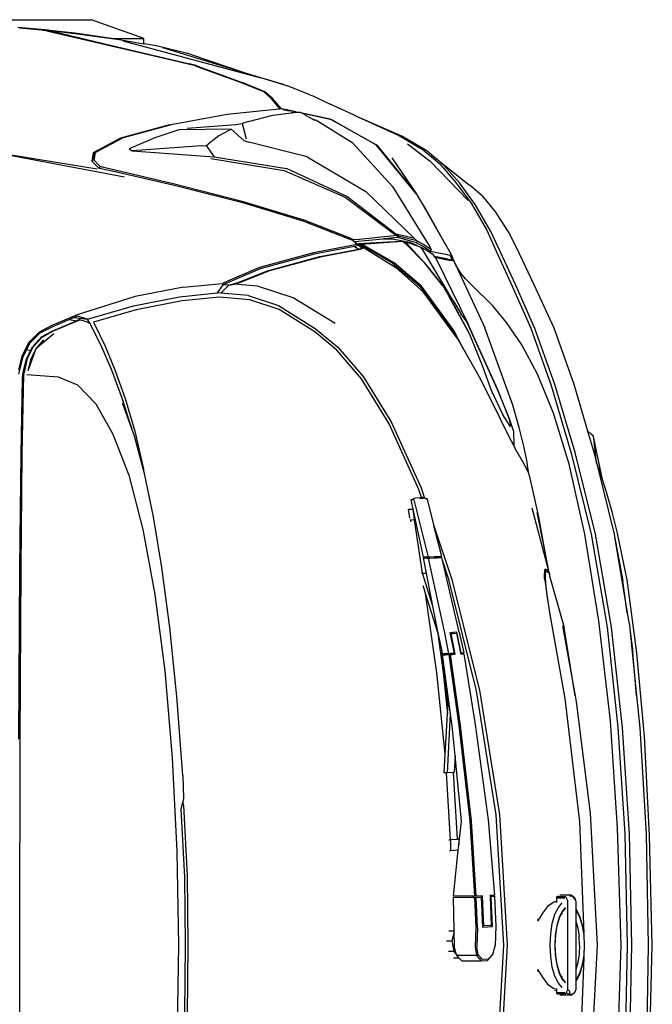
# Model space of a CAD drawing. Units: inches. Extents: x 22042254 to 25404563, y 17568978 to 17626777.
# Tile 18 of 45: x 22042342.8522 to 22042343.228, y 17568978.1821 to 17568978.767. Entities that reach past the tile are written whole.
import ezdxf

# ---------------------------------------------------------------- set-up
doc = ezdxf.new("R2010")
doc.units = ezdxf.units.IN
doc.header["$MEASUREMENT"] = 0
doc.layers.add('A-SITE-VEHI', color=8, linetype='Continuous', lineweight=18)
doc.layers.add('Edges', color=250, linetype='Continuous')

# ---------------------------------------------------------------- blocks, each defined once
blk = doc.blocks.new('Nissan Qashqai pl')
at = {"layer": 'Edges'}
for p, q in [((11.05972, 12.11965), (11.05938, 11.92208)), ((11.5166, 12.04708), (11.52386, 11.92208)), ((11.52698, 11.92208), (11.51964, 12.0475)), ((11.61327, 11.92208), (11.60675, 12.04892)), ((11.60051, 11.93346), (11.59629, 12.04057)), ((11.63292, 12.0344), (11.63628, 11.92208)), ((11.64211, 11.92208), (11.63993, 12.02899)), ((11.64437, 12.02886), (11.64655, 11.92208)), ((11.66226, 11.92208), (11.66041, 12.02874)), ((11.66349, 12.02738), (11.66628, 11.92208)), ((11.21164, 11.92208), (11.21014, 12.01197)), ((11.22044, 11.98904), (11.22108, 11.92208)), ((11.21801, 11.92208), (11.21745, 11.98742)), ((11.57617, 11.96938), (11.57479, 11.96843)), ((11.58846, 11.97008), (11.57758, 11.97008)), ((11.58668, 11.96947), (11.58377, 11.96782)), ((11.58679, 11.96604), (11.58668, 11.96947)), ((11.58961, 11.96947), (11.58668, 11.96947)), ((11.58846, 11.97008), (11.58961, 11.96947)), ((11.5915, 11.96782), (11.58961, 11.96947)), ((11.56588, 11.95938), (11.57195, 11.96347)), ((11.57195, 11.96347), (11.57457, 11.96395)), ((11.57261, 11.96533), (11.57261, 11.96561)), ((11.57306, 11.96528), (11.57306, 11.96569)), ((11.57479, 11.96843), (11.57457, 11.96768)), ((11.58239, 11.96768), (11.57457, 11.96768)), ((11.57457, 11.96768), (11.57457, 11.96395)), ((11.57457, 11.96395), (11.57457, 11.96378)), ((11.57479, 11.96843), (11.58262, 11.96843)), ((11.57994, 11.96265), (11.57613, 11.95845)), ((11.58262, 11.96843), (11.58377, 11.96782)), ((11.58377, 11.96782), (11.58513, 11.96453)), ((11.58679, 11.96604), (11.58513, 11.96453)), ((11.58513, 11.96453), (11.58513, 11.87963)), ((11.5915, 11.96782), (11.59043, 11.96839)), ((11.59285, 11.96453), (11.5915, 11.96782)), ((11.59285, 11.95694), (11.59285, 11.96453)), ((11.55816, 11.94815), (11.56082, 11.95281)), ((11.56082, 11.95281), (11.56588, 11.95938)), ((11.57286, 11.95178), (11.57035, 11.94308)), ((11.57613, 11.95845), (11.57286, 11.95178)), ((11.57692, 11.94885), (11.57987, 11.95487)), ((11.57876, 11.95169), (11.57712, 11.94834)), ((11.58001, 11.95424), (11.57876, 11.95169)), ((11.57876, 11.95169), (11.57995, 11.953)), ((11.57987, 11.95487), (11.58291, 11.95821)), ((11.58291, 11.95743), (11.58001, 11.95424)), ((11.59285, 11.95694), (11.59412, 11.95487)), ((11.59285, 11.95657), (11.59285, 11.95694)), ((11.59319, 11.9559), (11.59285, 11.95657)), ((11.59285, 11.95626), (11.59285, 11.95657)), ((11.59285, 11.95626), (11.59319, 11.9559)), ((11.59285, 11.95549), (11.59285, 11.95626)), ((11.59398, 11.95424), (11.59285, 11.95549)), ((11.59285, 11.94526), (11.59285, 11.95549)), ((11.59319, 11.9559), (11.59412, 11.95487)), ((11.59688, 11.94834), (11.59398, 11.95424)), ((11.59412, 11.95487), (11.59707, 11.94885)), ((11.55654, 11.94509), (11.55639, 11.94749)), ((11.55654, 11.94509), (11.55816, 11.94815)), ((11.57035, 11.94308), (11.56877, 11.93295)), ((11.57324, 11.93188), (11.57466, 11.94101)), ((11.5749, 11.94065), (11.5735, 11.93169)), ((11.57466, 11.94101), (11.57692, 11.94885)), ((11.57712, 11.94834), (11.5749, 11.94065)), ((11.59285, 11.8989), (11.59285, 11.94526)), ((11.59478, 11.93858), (11.59285, 11.94526)), ((11.5991, 11.94065), (11.59688, 11.94834)), ((11.59707, 11.94885), (11.59933, 11.94101)), ((11.60049, 11.93169), (11.5991, 11.94065)), ((11.59933, 11.94101), (11.60051, 11.93346)), ((11.48106, 11.93457), (11.47554, 11.93456)), ((11.47578, 11.92803), (11.4784, 11.93124)), ((11.4784, 11.93124), (11.47657, 11.92368)), ((11.4786, 11.93206), (11.4784, 11.93124)), ((11.48106, 11.93457), (11.4786, 11.93206)), ((11.49744, 11.93207), (11.4786, 11.93206)), ((11.48349, 11.93703), (11.48106, 11.93457)), ((11.48349, 11.93703), (11.50222, 11.93704)), ((11.49621, 11.92369), (11.49744, 11.93207)), ((11.49744, 11.93207), (11.50222, 11.93704)), ((11.49907, 11.93132), (11.49795, 11.92364)), ((11.50349, 11.93588), (11.49907, 11.93132)), ((11.50222, 11.93704), (11.50812, 11.93671)), ((11.50889, 11.93558), (11.50349, 11.93588)), ((11.50812, 11.93671), (11.51287, 11.9312)), ((11.50889, 11.93558), (11.51321, 11.93053)), ((11.51321, 11.93053), (11.51287, 11.9312)), ((11.56877, 11.93295), (11.56823, 11.92208)), ((11.57275, 11.92208), (11.57324, 11.93188)), ((11.5735, 11.93169), (11.57302, 11.92208)), ((11.59602, 11.93062), (11.59478, 11.93858)), ((11.60097, 11.92208), (11.60049, 11.93169)), ((11.60051, 11.93346), (11.60076, 11.93188)), ((11.60076, 11.93188), (11.60124, 11.92208)), ((11.05938, 11.92208), (11.05972, 11.72451)), ((11.21014, 11.8322), (11.21164, 11.92208)), ((11.21745, 11.85674), (11.21801, 11.92208)), ((11.22108, 11.92208), (11.22044, 11.85512)), ((11.47578, 11.92803), (11.47062, 11.92803)), ((11.47398, 11.91798), (11.47578, 11.92803)), ((11.47657, 11.92368), (11.47622, 11.90912)), ((11.49689, 11.90495), (11.49621, 11.92369)), ((11.49859, 11.9049), (11.49795, 11.92364)), ((11.51321, 11.93053), (11.51543, 11.92267)), ((11.51606, 11.90392), (11.51543, 11.92267)), ((11.52386, 11.92208), (11.5166, 11.79708)), ((11.51964, 11.79666), (11.52698, 11.92208)), ((11.56823, 11.92208), (11.56877, 11.91121)), ((11.57324, 11.91228), (11.57275, 11.92208)), ((11.57302, 11.92208), (11.5735, 11.91247)), ((11.59645, 11.92208), (11.59602, 11.93062)), ((11.59645, 11.92208), (11.59602, 11.91354)), ((11.60049, 11.91247), (11.60097, 11.92208)), ((11.60124, 11.92208), (11.60076, 11.91228)), ((11.60675, 11.79524), (11.61327, 11.92208)), ((11.63628, 11.92208), (11.63292, 11.80976)), ((11.63993, 11.81518), (11.64211, 11.92208)), ((11.64655, 11.92208), (11.64437, 11.8153)), ((11.66041, 11.81542), (11.66226, 11.92208)), ((11.66628, 11.92208), (11.66349, 11.81678)), ((11.46896, 11.91798), (11.47398, 11.91798)), ((11.47622, 11.90912), (11.47398, 11.91798)), ((11.57466, 11.90315), (11.57324, 11.91228)), ((11.5735, 11.91247), (11.5749, 11.90351)), ((11.59478, 11.90558), (11.59602, 11.91354)), ((11.5991, 11.90351), (11.60049, 11.91247)), ((11.60076, 11.91228), (11.60051, 11.91071)), ((11.47102, 11.90825), (11.4762, 11.90826)), ((11.4762, 11.90826), (11.47542, 11.87608)), ((11.47622, 11.90912), (11.4762, 11.90826)), ((11.49565, 11.87616), (11.49689, 11.90495)), ((11.49859, 11.9049), (11.49735, 11.87612)), ((11.50223, 11.8759), (11.50346, 11.90468)), ((11.50462, 11.90341), (11.50341, 11.87505)), ((11.50346, 11.90468), (11.51299, 11.90415)), ((11.51177, 11.90301), (11.50462, 11.90341)), ((11.51058, 11.87508), (11.51177, 11.90301)), ((11.51299, 11.90415), (11.51176, 11.87537)), ((11.51483, 11.87514), (11.51606, 11.90392)), ((11.56877, 11.91121), (11.57035, 11.90108)), ((11.57692, 11.89531), (11.57466, 11.90315)), ((11.5749, 11.90351), (11.57712, 11.89582)), ((11.59285, 11.8989), (11.59478, 11.90558)), ((11.59629, 11.80359), (11.60051, 11.91071)), ((11.59688, 11.89582), (11.5991, 11.90351)), ((11.59933, 11.90315), (11.59707, 11.89531)), ((11.60051, 11.91071), (11.59933, 11.90315)), ((11.55639, 11.89667), (11.55654, 11.89907)), ((11.55816, 11.89601), (11.55654, 11.89907)), ((11.56082, 11.89135), (11.55816, 11.89601)), ((11.57035, 11.90108), (11.57286, 11.89238)), ((11.57987, 11.88929), (11.57692, 11.89531)), ((11.57712, 11.89582), (11.57876, 11.89248)), ((11.59285, 11.88868), (11.59285, 11.8989)), ((11.59398, 11.88992), (11.59688, 11.89582)), ((11.59707, 11.89531), (11.59412, 11.88929)), ((11.56588, 11.88478), (11.56082, 11.89135)), ((11.57195, 11.88069), (11.56588, 11.88478)), ((11.57286, 11.89238), (11.57613, 11.88571)), ((11.57613, 11.88571), (11.57994, 11.88151)), ((11.57995, 11.89116), (11.57876, 11.89248)), ((11.57876, 11.89248), (11.58001, 11.88992)), ((11.58291, 11.88595), (11.57987, 11.88929)), ((11.58001, 11.88992), (11.58291, 11.88673)), ((11.59285, 11.88868), (11.59398, 11.88992)), ((11.59285, 11.88722), (11.59412, 11.88929)), ((11.59285, 11.8879), (11.59285, 11.88868)), ((11.59285, 11.88759), (11.59319, 11.88827)), ((11.59319, 11.88827), (11.59285, 11.8879)), ((11.59285, 11.88759), (11.59285, 11.8879)), ((11.59285, 11.88722), (11.59285, 11.88759)), ((11.59285, 11.87963), (11.59285, 11.88722)), ((11.59412, 11.88929), (11.59319, 11.88827)), ((11.49563, 11.87496), (11.47539, 11.87488)), ((11.47539, 11.87488), (11.4801, 11.83099)), ((11.47542, 11.87608), (11.49451, 11.87616)), ((11.49133, 11.80278), (11.49563, 11.87496)), ((11.49732, 11.87492), (11.49295, 11.80271)), ((11.49449, 11.87502), (11.49451, 11.87616)), ((11.50341, 11.87505), (11.49449, 11.87502)), ((11.49451, 11.87616), (11.49565, 11.87616)), ((11.49732, 11.87492), (11.49563, 11.87496)), ((11.49565, 11.87616), (11.49735, 11.87612)), ((11.50339, 11.87463), (11.49732, 11.87492)), ((11.49735, 11.87612), (11.50223, 11.8759)), ((11.50341, 11.87505), (11.50339, 11.87463)), ((11.51054, 11.87423), (11.51058, 11.87508)), ((11.51472, 11.8751), (11.51058, 11.87508)), ((11.51176, 11.87537), (11.51472, 11.87515)), ((11.51472, 11.87515), (11.51472, 11.8751)), ((11.51472, 11.87515), (11.51483, 11.87514)), ((11.51483, 11.87514), (11.51472, 11.8751)), ((11.57261, 11.88057), (11.57195, 11.88069)), ((11.57261, 11.88057), (11.57261, 11.88076)), ((11.57306, 11.88049), (11.57261, 11.88057)), ((11.57306, 11.88049), (11.57306, 11.88081)), ((11.57457, 11.88021), (11.57306, 11.88049)), ((11.57457, 11.88096), (11.57457, 11.88021)), ((11.57457, 11.88021), (11.57457, 11.87648)), ((11.57457, 11.87648), (11.58239, 11.87648)), ((11.57457, 11.87648), (11.57479, 11.87573)), ((11.58262, 11.87573), (11.57479, 11.87573)), ((11.57479, 11.87573), (11.57617, 11.87478)), ((11.58377, 11.87635), (11.58262, 11.87573)), ((11.58513, 11.87963), (11.58377, 11.87635)), ((11.58668, 11.87469), (11.58961, 11.87469)), ((11.58961, 11.87469), (11.58846, 11.87408)), ((11.58961, 11.87469), (11.5915, 11.87635)), ((11.59043, 11.87577), (11.58961, 11.87469)), ((11.59221, 11.87812), (11.59043, 11.87577)), ((11.59043, 11.87577), (11.5915, 11.87635)), ((11.5915, 11.87635), (11.59221, 11.87812)), ((11.59285, 11.87963), (11.59221, 11.87812)), ((11.50884, 11.80182), (11.5148, 11.87394)), ((11.5148, 11.87394), (11.51054, 11.87423)), ((11.58846, 11.87408), (11.57758, 11.87408)), ((11.2139, 11.7914), (11.21745, 11.85674)), ((11.22044, 11.85512), (11.21682, 11.78816)), ((11.20565, 11.74231), (11.21014, 11.8322)), ((11.47305, 11.83139), (11.47165, 11.83144)), ((11.47305, 11.83139), (11.473, 11.82087)), ((11.4801, 11.83099), (11.47305, 11.83139)), ((11.4801, 11.83099), (11.48065, 11.82584)), ((11.47281, 11.82086), (11.46872, 11.75675)), ((11.47111, 11.82093), (11.47189, 11.82089)), ((11.47281, 11.82086), (11.47189, 11.82089)), ((11.473, 11.82087), (11.47281, 11.82086)), ((11.47916, 11.8205), (11.473, 11.82087)), ((11.47508, 11.75641), (11.47919, 11.82046)), ((11.47919, 11.82046), (11.47916, 11.8205)), ((11.48062, 11.82044), (11.47919, 11.82046)), ((11.48062, 11.82044), (11.48065, 11.82584)), ((11.48065, 11.82584), (11.4831, 11.803)), ((11.63292, 11.80976), (11.62604, 11.70665)), ((11.63327, 11.71316), (11.63993, 11.81518)), ((11.64437, 11.8153), (11.63768, 11.7134)), ((11.65425, 11.71357), (11.66041, 11.81542)), ((11.66349, 11.81678), (11.65888, 11.72193)), ((11.4831, 11.803), (11.47707, 11.74042)), ((11.4805, 11.71128), (11.49133, 11.80278)), ((11.49295, 11.80271), (11.48212, 11.71121)), ((11.49642, 11.71041), (11.50884, 11.80182)), ((11.58235, 11.68521), (11.59629, 11.80359)), ((11.21579, 11.78424), (11.2139, 11.7914)), ((11.5166, 11.79708), (11.49761, 11.67796)), ((11.50045, 11.6772), (11.51964, 11.79666)), ((11.5932, 11.68852), (11.60675, 11.79524)), ((11.21682, 11.78816), (11.21579, 11.78424)), ((11.21585, 11.78401), (11.21579, 11.78424)), ((11.21682, 11.78816), (11.21585, 11.78401)), ((11.21658, 11.78121), (11.21585, 11.78401)), ((11.21586, 11.75915), (11.21658, 11.78121)), ((11.21586, 11.75915), (11.20997, 11.68347)), ((11.46872, 11.75675), (11.46649, 11.75682)), ((11.46649, 11.75682), (11.46757, 11.73891)), ((11.46975, 11.75671), (11.46872, 11.75675)), ((11.46975, 11.75671), (11.47273, 11.69994)), ((11.47508, 11.75641), (11.46975, 11.75671)), ((11.47611, 11.75636), (11.47508, 11.75641)), ((11.47707, 11.74042), (11.47611, 11.75636)), ((11.19842, 11.65867), (11.20565, 11.74231)), ((11.46757, 11.73891), (11.45941, 11.6607)), ((11.46757, 11.73891), (11.46992, 11.70014)), ((11.47707, 11.74042), (11.47428, 11.71144)), ((11.0586, 11.72441), (11.05947, 11.55994)), ((11.05972, 11.72451), (11.06059, 11.56009)), ((11.65888, 11.72193), (11.65143, 11.64152)), ((11.47094, 11.64327), (11.4805, 11.71128)), ((11.48212, 11.71121), (11.47257, 11.6432)), ((11.47428, 11.71144), (11.47273, 11.69994)), ((11.48539, 11.64249), (11.49642, 11.71041)), ((11.62604, 11.70665), (11.61495, 11.61084)), ((11.6229, 11.61679), (11.63327, 11.71316)), ((11.63768, 11.7134), (11.62719, 11.61693)), ((11.65114, 11.68233), (11.65425, 11.71357)), ((11.47273, 11.69994), (11.46512, 11.64343)), ((11.46576, 11.66035), (11.46992, 11.70014)), ((11.46992, 11.70014), (11.47047, 11.69095)), ((11.47047, 11.69095), (11.46419, 11.63849)), ((11.59218, 11.68277), (11.5932, 11.68852)), ((11.20997, 11.68347), (11.2033, 11.61723)), ((11.49761, 11.67796), (11.47115, 11.57128)), ((11.47375, 11.5702), (11.50045, 11.6772)), ((11.56846, 11.60829), (11.58235, 11.68521)), ((11.58021, 11.61555), (11.59218, 11.68277)), ((11.59218, 11.68277), (11.58179, 11.61717)), ((11.64478, 11.61839), (11.65114, 11.68233)), ((11.65114, 11.68233), (11.64749, 11.64092)), ((11.18907, 11.58559), (11.19842, 11.65867)), ((11.45941, 11.6607), (11.44866, 11.58459)), ((11.46024, 11.62121), (11.46576, 11.66035)), ((11.46419, 11.63849), (11.46114, 11.62406)), ((11.46505, 11.64255), (11.46419, 11.63849)), ((11.46792, 11.64248), (11.46505, 11.64255)), ((11.46512, 11.64343), (11.46801, 11.64335)), ((11.46687, 11.62247), (11.47088, 11.64239)), ((11.46801, 11.64335), (11.46792, 11.64248)), ((11.47088, 11.64239), (11.46792, 11.64248)), ((11.46801, 11.64335), (11.47094, 11.64327)), ((11.47252, 11.64233), (11.47088, 11.64239)), ((11.47094, 11.64327), (11.47257, 11.6432)), ((11.47212, 11.62223), (11.47625, 11.64214)), ((11.47439, 11.64223), (11.47252, 11.64233)), ((11.47257, 11.6432), (11.47449, 11.6431)), ((11.47727, 11.64296), (11.47315, 11.62305)), ((11.47439, 11.64223), (11.47449, 11.6431)), ((11.47625, 11.64214), (11.47439, 11.64223)), ((11.47449, 11.6431), (11.47727, 11.64296)), ((11.47827, 11.62277), (11.48226, 11.64167)), ((11.48298, 11.64165), (11.47879, 11.62186)), ((11.48098, 11.62171), (11.48532, 11.64161)), ((11.48226, 11.64167), (11.48244, 11.64254)), ((11.48226, 11.64167), (11.48298, 11.64165)), ((11.48244, 11.64254), (11.48247, 11.64267)), ((11.48535, 11.64246), (11.48244, 11.64254)), ((11.48247, 11.64267), (11.48535, 11.64246)), ((11.483, 11.64176), (11.48298, 11.64165)), ((11.48532, 11.64161), (11.483, 11.64176)), ((11.48539, 11.64249), (11.48535, 11.64246)), ((11.65143, 11.64152), (11.64217, 11.57162)), ((11.64478, 11.61839), (11.64749, 11.64092)), ((11.46024, 11.62121), (11.44866, 11.58459)), ((11.45125, 11.55073), (11.46687, 11.62247)), ((11.46083, 11.62261), (11.45585, 11.5969)), ((11.46114, 11.62406), (11.46024, 11.62121)), ((11.46114, 11.62406), (11.46083, 11.62261)), ((11.48098, 11.62171), (11.4649, 11.55261)), ((11.47495, 11.62207), (11.47212, 11.62223)), ((11.47315, 11.62305), (11.47515, 11.62294)), ((11.47495, 11.62207), (11.47515, 11.62294)), ((11.47879, 11.62186), (11.47495, 11.62207)), ((11.47515, 11.62294), (11.47827, 11.62277)), ((11.2033, 11.61723), (11.19582, 11.55976)), ((11.56776, 11.56755), (11.58179, 11.61717)), ((11.61495, 11.61084), (11.6016, 11.52761)), ((11.60765, 11.5276), (11.6229, 11.61679)), ((11.62719, 11.61693), (11.61178, 11.52762)), ((11.64227, 11.603), (11.64462, 11.61709)), ((11.64462, 11.61709), (11.64478, 11.61839)), ((11.56499, 11.58644), (11.56846, 11.60829)), ((11.56905, 11.60888), (11.56563, 11.58822)), ((11.63012, 11.53004), (11.64227, 11.603)), ((11.64227, 11.603), (11.63807, 11.5726)), ((11.45585, 11.5969), (11.44582, 11.56516)), ((11.45585, 11.5969), (11.44965, 11.56495)), ((11.17758, 11.52307), (11.18907, 11.58559)), ((11.44866, 11.58459), (11.44723, 11.58007)), ((11.56356, 11.57357), (11.56499, 11.58644)), ((11.56563, 11.58822), (11.56415, 11.57536)), ((11.44723, 11.58007), (11.44639, 11.57739)), ((11.56335, 11.56843), (11.56356, 11.57357)), ((11.56415, 11.57536), (11.56375, 11.56794)), ((11.63012, 11.53004), (11.63807, 11.5726)), ((11.44575, 11.56516), (11.43801, 11.51398)), ((11.4448, 11.5652), (11.44575, 11.56516)), ((11.44575, 11.56516), (11.44582, 11.56516)), ((11.44582, 11.56516), (11.44965, 11.56495)), ((11.44965, 11.56495), (11.44685, 11.5505)), ((11.45676, 11.51971), (11.47375, 11.5702)), ((11.47115, 11.57128), (11.4649, 11.55261)), ((11.56255, 11.56701), (11.56268, 11.56956)), ((11.56271, 11.56245), (11.56255, 11.56701)), ((11.56268, 11.56956), (11.56259, 11.5697)), ((11.56268, 11.56956), (11.5628, 11.57206)), ((11.56335, 11.56843), (11.56268, 11.56956)), ((11.56325, 11.56586), (11.56335, 11.56843)), ((11.56334, 11.56271), (11.56325, 11.56586)), ((11.56609, 11.56386), (11.56334, 11.56271)), ((11.56368, 11.56788), (11.56335, 11.56843)), ((11.56375, 11.56794), (11.56392, 11.56325)), ((11.56392, 11.56325), (11.56429, 11.56338)), ((11.56429, 11.56338), (11.56596, 11.56408)), ((11.56487, 11.5659), (11.56469, 11.5662)), ((11.56609, 11.56386), (11.56583, 11.56223)), ((11.56596, 11.56408), (11.56616, 11.56417)), ((11.56609, 11.56386), (11.56596, 11.56408)), ((11.56613, 11.56388), (11.56609, 11.56386)), ((11.56618, 11.56418), (11.56613, 11.56388)), ((11.56613, 11.56388), (11.56616, 11.56417)), ((11.56613, 11.56388), (11.56645, 11.5641)), ((11.56665, 11.56424), (11.56616, 11.56236)), ((11.56616, 11.56417), (11.56618, 11.56418)), ((11.56616, 11.56236), (11.56645, 11.5641)), ((11.56618, 11.56418), (11.56648, 11.56431)), ((11.56645, 11.5641), (11.56648, 11.56431)), ((11.56645, 11.5641), (11.56665, 11.56424)), ((11.56648, 11.56431), (11.56669, 11.5644)), ((11.56661, 11.56253), (11.56704, 11.56455)), ((11.56665, 11.56424), (11.56688, 11.56448)), ((11.56669, 11.5644), (11.56665, 11.56424)), ((11.56669, 11.5644), (11.56688, 11.56448)), ((11.56671, 11.56257), (11.56712, 11.56458)), ((11.56717, 11.5646), (11.56679, 11.56261)), ((11.56688, 11.56448), (11.56704, 11.56455)), ((11.56704, 11.56455), (11.56739, 11.56625)), ((11.56704, 11.56455), (11.56712, 11.56458)), ((11.56712, 11.56458), (11.56763, 11.56708)), ((11.56712, 11.56458), (11.56717, 11.5646)), ((11.56717, 11.5646), (11.56763, 11.56708)), ((11.56745, 11.56646), (11.56739, 11.56625)), ((11.56763, 11.56708), (11.56776, 11.56755)), ((11.64217, 11.57162), (11.63751, 11.54857)), ((11.05947, 11.55994), (11.06074, 11.45082)), ((11.06059, 11.56009), (11.06182, 11.4509)), ((11.19582, 11.55976), (11.18773, 11.51111)), ((11.55053, 11.5023), (11.56648, 11.56144)), ((11.56334, 11.56271), (11.56271, 11.56245)), ((11.56338, 11.56129), (11.56271, 11.56245)), ((11.56273, 11.5431), (11.56648, 11.56144)), ((11.56338, 11.56129), (11.56334, 11.56271)), ((11.56583, 11.56223), (11.56338, 11.56129)), ((11.56616, 11.56236), (11.56583, 11.56223)), ((11.56661, 11.56253), (11.56616, 11.56236)), ((11.56679, 11.56261), (11.56648, 11.56144)), ((11.56671, 11.56257), (11.56661, 11.56253)), ((11.56679, 11.56261), (11.56671, 11.56257)), ((11.43747, 11.49463), (11.45125, 11.54985)), ((11.44684, 11.54963), (11.43914, 11.51392)), ((11.44983, 11.54978), (11.44684, 11.54963)), ((11.44685, 11.5505), (11.44997, 11.55066)), ((11.44983, 11.54978), (11.44997, 11.55066)), ((11.45125, 11.54985), (11.44983, 11.54978)), ((11.44997, 11.55066), (11.45125, 11.55073)), ((11.45125, 11.55073), (11.4529, 11.55066)), ((11.4529, 11.54978), (11.45125, 11.54985)), ((11.4529, 11.55066), (11.45711, 11.55045)), ((11.45711, 11.54958), (11.4529, 11.54978)), ((11.46429, 11.54915), (11.45676, 11.51971)), ((11.45711, 11.55045), (11.45994, 11.5503)), ((11.46197, 11.5493), (11.45711, 11.54958)), ((11.45983, 11.54978), (11.45994, 11.5503)), ((11.46402, 11.54999), (11.45983, 11.54978)), ((11.45994, 11.5503), (11.46197, 11.55018)), ((11.46197, 11.55018), (11.46404, 11.55004)), ((11.46375, 11.54918), (11.46197, 11.5493)), ((11.46402, 11.54999), (11.46375, 11.54918)), ((11.46429, 11.54915), (11.46375, 11.54918)), ((11.46404, 11.55004), (11.46402, 11.54999)), ((11.46423, 11.55), (11.46402, 11.54999)), ((11.46404, 11.55004), (11.46423, 11.55)), ((11.46423, 11.55), (11.46424, 11.55003)), ((11.4643, 11.55002), (11.46423, 11.55)), ((11.4649, 11.55261), (11.4643, 11.55002)), ((11.63751, 11.54857), (11.63276, 11.52672)), ((11.55533, 11.50682), (11.56273, 11.5431)), ((11.55707, 11.51104), (11.56273, 11.5431)), ((11.6016, 11.52761), (11.58664, 11.46068)), ((11.58843, 11.44985), (11.60765, 11.5276)), ((11.61178, 11.52762), (11.59225, 11.44945)), ((11.61272, 11.45895), (11.62966, 11.52759)), ((11.63276, 11.52672), (11.62771, 11.50627)), ((11.62966, 11.52759), (11.63012, 11.53004)), ((11.16395, 11.47112), (11.17758, 11.52307)), ((11.43501, 11.51584), (11.43475, 11.51409)), ((11.45032, 11.49453), (11.45676, 11.51971)), ((11.18773, 11.51111), (11.17906, 11.46956)), ((11.43371, 11.51238), (11.43251, 11.50378)), ((11.43475, 11.51409), (11.43403, 11.51411)), ((11.43801, 11.51398), (11.43475, 11.51409)), ((11.4382, 11.51397), (11.43676, 11.50364)), ((11.43914, 11.51392), (11.43692, 11.50363)), ((11.4382, 11.51397), (11.43801, 11.51398)), ((11.43914, 11.51392), (11.4382, 11.51397)), ((11.54814, 11.47101), (11.55707, 11.51104)), ((11.62771, 11.50627), (11.62241, 11.48743)), ((11.43251, 11.50378), (11.43676, 11.50364)), ((11.43251, 11.50378), (11.4369, 11.50353)), ((11.4369, 11.50353), (11.435, 11.49469)), ((11.43676, 11.50364), (11.43692, 11.50363)), ((11.43692, 11.50363), (11.4369, 11.50353)), ((11.435, 11.49469), (11.43896, 11.49272)), ((11.43747, 11.49463), (11.435, 11.49469)), ((11.43896, 11.49272), (11.44373, 11.49245)), ((11.44474, 11.49242), (11.44218, 11.48476)), ((11.44507, 11.49341), (11.44316, 11.49351)), ((11.44373, 11.49245), (11.44491, 11.49291)), ((11.44474, 11.49242), (11.44373, 11.49245)), ((11.44453, 11.48334), (11.44778, 11.49299)), ((11.44491, 11.49291), (11.44474, 11.49242)), ((11.4462, 11.49239), (11.44474, 11.49242)), ((11.44507, 11.49341), (11.44491, 11.49291)), ((11.44491, 11.49291), (11.44606, 11.49335)), ((11.44606, 11.49335), (11.44507, 11.49341)), ((11.44786, 11.49325), (11.44606, 11.49335)), ((11.44786, 11.49325), (11.4462, 11.49239)), ((11.44778, 11.49299), (11.4462, 11.49239)), ((11.45018, 11.49392), (11.44778, 11.49299)), ((11.44794, 11.49325), (11.44786, 11.49325)), ((11.45032, 11.49453), (11.44794, 11.49325)), ((11.45018, 11.49392), (11.45032, 11.49453)), ((11.62241, 11.48743), (11.61848, 11.47528)), ((11.44218, 11.48476), (11.41383, 11.42186)), ((11.41588, 11.41997), (11.44453, 11.48334)), ((11.14869, 11.43161), (11.16395, 11.47112)), ((11.17906, 11.46956), (11.17808, 11.46592)), ((11.54554, 11.46484), (11.54721, 11.46841)), ((11.54814, 11.47101), (11.54666, 11.46197)), ((11.61848, 11.47528), (11.61008, 11.43562)), ((11.61742, 11.47198), (11.61272, 11.45895)), ((11.61848, 11.47528), (11.61742, 11.47198)), ((11.17808, 11.46592), (11.1694, 11.43374)), ((11.1699, 11.42889), (11.17797, 11.4652)), ((11.17797, 11.4652), (11.17808, 11.46592)), ((11.54162, 11.45783), (11.54554, 11.46484)), ((11.54666, 11.46197), (11.54611, 11.45874)), ((11.58664, 11.46068), (11.57152, 11.41151)), ((11.61272, 11.45895), (11.61008, 11.43562)), ((11.61028, 11.44915), (11.61272, 11.45895)), ((11.06074, 11.45082), (11.06214, 11.37845)), ((11.06182, 11.4509), (11.06324, 11.37414)), ((11.53572, 11.44731), (11.54162, 11.45783)), ((11.54611, 11.45874), (11.54336, 11.44449)), ((11.56912, 11.38501), (11.58843, 11.44985)), ((11.59225, 11.44945), (11.57263, 11.38419)), ((11.52833, 11.43321), (11.53335, 11.4428)), ((11.53261, 11.43965), (11.5333, 11.44225)), ((11.53313, 11.42848), (11.53354, 11.44315)), ((11.5333, 11.44225), (11.53335, 11.4428)), ((11.53335, 11.4428), (11.53354, 11.44315)), ((11.53354, 11.44315), (11.53572, 11.44731)), ((11.54336, 11.44449), (11.53855, 11.42543)), ((11.60419, 11.42861), (11.61028, 11.44915)), ((11.1323, 11.40268), (11.14869, 11.43161)), ((11.1694, 11.43374), (11.1668, 11.42651)), ((11.5202, 11.41712), (11.52833, 11.43321)), ((11.60772, 11.43162), (11.60419, 11.42861)), ((11.60938, 11.43347), (11.60772, 11.43162)), ((11.61008, 11.43562), (11.60938, 11.43347)), ((11.1668, 11.42651), (11.1582, 11.40259)), ((11.16047, 11.39766), (11.1699, 11.42889)), ((11.16426, 11.41918), (11.1668, 11.42651)), ((11.41383, 11.42186), (11.38718, 11.37878)), ((11.53009, 11.42439), (11.52299, 11.41307)), ((11.52855, 11.41625), (11.53022, 11.42324)), ((11.53313, 11.42848), (11.52922, 11.417)), ((11.53022, 11.42324), (11.53009, 11.42439)), ((11.53855, 11.42543), (11.53253, 11.4038)), ((11.59084, 11.38361), (11.60419, 11.42861)), ((11.15764, 11.39828), (11.16426, 11.41918)), ((11.15766, 11.39771), (11.16426, 11.41918)), ((11.16426, 11.41918), (11.15826, 11.40186)), ((11.38877, 11.37638), (11.41588, 11.41997)), ((11.50131, 11.37908), (11.5202, 11.41712)), ((11.5118, 11.38938), (11.52299, 11.41307)), ((11.52922, 11.417), (11.51787, 11.38901)), ((11.51787, 11.38901), (11.52855, 11.41625)), ((11.11477, 11.38434), (11.1323, 11.40268)), ((11.53253, 11.4038), (11.50574, 11.32965)), ((11.57152, 11.41151), (11.55624, 11.37411)), ((11.14751, 11.37001), (11.15766, 11.39771)), ((11.15051, 11.36998), (11.16047, 11.39766)), ((11.5118, 11.38938), (11.51304, 11.39274)), ((11.09618, 11.37663), (11.11477, 11.38434)), ((11.51787, 11.38901), (11.48801, 11.32337)), ((11.49005, 11.3275), (11.51787, 11.38901)), ((11.50277, 11.36495), (11.5118, 11.38938)), ((11.54963, 11.33002), (11.56912, 11.38501)), ((11.57263, 11.38419), (11.5535, 11.33028)), ((11.57164, 11.32969), (11.59084, 11.38361)), ((11.06236, 11.3576), (11.05822, 11.37418)), ((11.06214, 11.37845), (11.06222, 11.37449)), ((11.06222, 11.37449), (11.06303, 11.37135)), ((11.06324, 11.37414), (11.06408, 11.37085)), ((11.06624, 11.37435), (11.09618, 11.37663)), ((11.38718, 11.37878), (11.3635, 11.35125)), ((11.36451, 11.34835), (11.38877, 11.37638)), ((11.48518, 11.35017), (11.50131, 11.37908)), ((11.55624, 11.37411), (11.54097, 11.34593)), ((11.06139, 11.35691), (11.05807, 11.37037)), ((11.06303, 11.37135), (11.06594, 11.3594)), ((11.06408, 11.37085), (11.06692, 11.35921)), ((11.06961, 11.36056), (11.0671, 11.37109)), ((11.07472, 11.34981), (11.0671, 11.37109)), ((11.13692, 11.34555), (11.14751, 11.37001)), ((11.14123, 11.34726), (11.15051, 11.36998)), ((11.49086, 11.33567), (11.50277, 11.36495)), ((11.06818, 11.34377), (11.06139, 11.35691)), ((11.06584, 11.35092), (11.06236, 11.3576)), ((11.06594, 11.3594), (11.06978, 11.35164)), ((11.06692, 11.35921), (11.0727, 11.34754)), ((11.07472, 11.34981), (11.06961, 11.36056)), ((11.06978, 11.35164), (11.06584, 11.35092)), ((11.06918, 11.34452), (11.06584, 11.35092)), ((11.06978, 11.35164), (11.07183, 11.3475)), ((11.07183, 11.3475), (11.08018, 11.33842)), ((11.0727, 11.34754), (11.0809, 11.33858)), ((11.08206, 11.34125), (11.07472, 11.34981)), ((11.092, 11.33548), (11.07472, 11.34981)), ((11.12767, 11.32749), (11.13692, 11.34555)), ((11.13017, 11.32416), (11.14123, 11.34726)), ((11.3635, 11.35125), (11.34251, 11.3336)), ((11.34283, 11.33026), (11.36451, 11.34835)), ((11.48518, 11.35017), (11.4758, 11.33232)), ((11.48012, 11.34111), (11.48518, 11.35017)), ((11.54097, 11.34593), (11.52646, 11.32473)), ((11.07787, 11.3339), (11.06818, 11.34377)), ((11.07866, 11.33492), (11.06918, 11.34452)), ((11.08018, 11.33842), (11.09121, 11.33249)), ((11.0809, 11.33858), (11.09174, 11.33271)), ((11.48005, 11.341), (11.44669, 11.29536)), ((11.47876, 11.33901), (11.47454, 11.33252)), ((11.47876, 11.33901), (11.48005, 11.341)), ((11.48005, 11.341), (11.48012, 11.34111)), ((11.09022, 11.32753), (11.07787, 11.3339)), ((11.09081, 11.32882), (11.07866, 11.33492)), ((11.11439, 11.31711), (11.09022, 11.32753)), ((11.10704, 11.32181), (11.09081, 11.32882)), ((11.09121, 11.33249), (11.1138, 11.3229)), ((11.09174, 11.33271), (11.11486, 11.323)), ((11.12645, 11.32495), (11.12767, 11.32749)), ((11.30757, 11.30833), (11.34283, 11.33026)), ((11.34251, 11.3336), (11.3082, 11.31215)), ((11.44331, 11.28988), (11.47454, 11.33252)), ((11.4758, 11.33232), (11.44474, 11.28965)), ((11.46332, 11.28473), (11.48966, 11.33337)), ((11.47038, 11.29841), (11.49086, 11.33567)), ((11.47038, 11.29841), (11.48966, 11.33337)), ((11.48133, 11.27727), (11.50574, 11.32965)), ((11.48983, 11.32694), (11.48954, 11.32636)), ((11.48966, 11.33337), (11.49086, 11.33567)), ((11.48983, 11.32694), (11.49005, 11.3275)), ((11.53062, 11.28691), (11.54963, 11.33002)), ((11.5535, 11.33028), (11.53487, 11.28826)), ((11.55274, 11.28821), (11.57164, 11.32969)), ((11.10704, 11.32181), (11.1138, 11.3229)), ((11.11164, 11.31982), (11.10704, 11.32181)), ((11.11164, 11.31982), (11.1244, 11.32146)), ((11.11467, 11.31851), (11.11164, 11.31982)), ((11.1138, 11.3229), (11.11393, 11.32284)), ((11.11393, 11.32284), (11.1164, 11.32172)), ((11.1244, 11.32146), (11.11467, 11.31851)), ((11.11486, 11.323), (11.1172, 11.32196)), ((11.1164, 11.32172), (11.1172, 11.32196)), ((11.11744, 11.32189), (11.1164, 11.32172)), ((11.1172, 11.32196), (11.11744, 11.32189)), ((11.11744, 11.32189), (11.11997, 11.32267)), ((11.11997, 11.32267), (11.12459, 11.32429)), ((11.12604, 11.32481), (11.1244, 11.32146)), ((11.1244, 11.32146), (11.12591, 11.32476)), ((11.1244, 11.32146), (11.16836, 11.30873)), ((11.12459, 11.32429), (11.12591, 11.32476)), ((11.12466, 11.32442), (11.12595, 11.32486)), ((11.12478, 11.32467), (11.12595, 11.32486)), ((11.12595, 11.32486), (11.1251, 11.3253)), ((11.12591, 11.32476), (11.12595, 11.32486)), ((11.12591, 11.32476), (11.12604, 11.32481)), ((11.12595, 11.32486), (11.12626, 11.32554)), ((11.12595, 11.32486), (11.12607, 11.32488)), ((11.12604, 11.32481), (11.12645, 11.32495)), ((11.12607, 11.32488), (11.12604, 11.32481)), ((11.12631, 11.32537), (11.12607, 11.32488)), ((11.12607, 11.32488), (11.12645, 11.32495)), ((11.17121, 11.31245), (11.13017, 11.32416)), ((11.36192, 11.32544), (11.32179, 11.30083)), ((11.45883, 11.26345), (11.48954, 11.32636)), ((11.48801, 11.32337), (11.48281, 11.31653)), ((11.52646, 11.32473), (11.51313, 11.30854)), ((11.17021, 11.29978), (11.11439, 11.31711)), ((11.16836, 11.30873), (11.21271, 11.29983)), ((11.21523, 11.3038), (11.17121, 11.31245)), ((11.27848, 11.29865), (11.30757, 11.30833)), ((11.3082, 11.31215), (11.28005, 11.30276)), ((11.47499, 11.30324), (11.48281, 11.31653)), ((11.51313, 11.30854), (11.49329, 11.28912)), ((11.21656, 11.2908), (11.17021, 11.29978)), ((11.21271, 11.29983), (11.24875, 11.29618)), ((11.2509, 11.3003), (11.21523, 11.3038)), ((11.28005, 11.30276), (11.2509, 11.3003)), ((11.27848, 11.29865), (11.25238, 11.29648)), ((11.32179, 11.30083), (11.28736, 11.28974)), ((11.47499, 11.30324), (11.4462, 11.25482)), ((11.47026, 11.29821), (11.47038, 11.29841)), ((11.21656, 11.2908), (11.25377, 11.28706)), ((11.25238, 11.29648), (11.24875, 11.29618)), ((11.2541, 11.28846), (11.24875, 11.29618)), ((11.25238, 11.29648), (11.25993, 11.28891)), ((11.25993, 11.28891), (11.2541, 11.28846)), ((11.25993, 11.28891), (11.25999, 11.28889)), ((11.25999, 11.28889), (11.26503, 11.28789)), ((11.25999, 11.28889), (11.26771, 11.28668)), ((11.28736, 11.28974), (11.27242, 11.28847)), ((11.41708, 11.26758), (11.44331, 11.28988)), ((11.44474, 11.28965), (11.41866, 11.26734)), ((11.42028, 11.27173), (11.44669, 11.29536)), ((11.44691, 11.26684), (11.46587, 11.29022)), ((11.46538, 11.28932), (11.44788, 11.2676)), ((11.46538, 11.28932), (11.46587, 11.29022)), ((11.46587, 11.29022), (11.46737, 11.29293)), ((11.46746, 11.29312), (11.46737, 11.29293)), ((11.46746, 11.29312), (11.47026, 11.29821)), ((11.49329, 11.28912), (11.48692, 11.28262)), ((11.25857, 11.28503), (11.25377, 11.28706)), ((11.29, 11.2731), (11.2541, 11.28846)), ((11.28951, 11.27177), (11.25857, 11.28503)), ((11.27242, 11.28847), (11.26503, 11.28789)), ((11.26503, 11.28789), (11.27055, 11.28622)), ((11.26771, 11.28668), (11.26785, 11.28663)), ((11.26785, 11.28663), (11.29721, 11.27493)), ((11.27055, 11.28622), (11.29928, 11.27468)), ((11.48692, 11.28262), (11.48256, 11.27724)), ((11.51652, 11.25601), (11.53062, 11.28691)), ((11.53487, 11.28826), (11.52058, 11.25724)), ((11.53843, 11.2583), (11.55274, 11.28821)), ((11.3411, 11.25789), (11.28951, 11.27177)), ((11.34188, 11.25916), (11.29, 11.2731)), ((11.29721, 11.27493), (11.34742, 11.26142)), ((11.29928, 11.27468), (11.34932, 11.2614)), ((11.39234, 11.25471), (11.42028, 11.27173)), ((11.47707, 11.26812), (11.48133, 11.27727)), ((11.48256, 11.27724), (11.47783, 11.26953)), ((11.48133, 11.27727), (11.48217, 11.27864)), ((11.34742, 11.26142), (11.38475, 11.2543)), ((11.34932, 11.2614), (11.38634, 11.25437)), ((11.41708, 11.26758), (11.38507, 11.24911)), ((11.41866, 11.26734), (11.3914, 11.25156)), ((11.42958, 11.2488), (11.44691, 11.26684)), ((11.44788, 11.2676), (11.43028, 11.24852)), ((11.45491, 11.25868), (11.45678, 11.26054)), ((11.4564, 11.26086), (11.45669, 11.26088)), ((11.45652, 11.26104), (11.45688, 11.26111)), ((11.45678, 11.26054), (11.45714, 11.2609)), ((11.45714, 11.2609), (11.45732, 11.2612)), ((11.45729, 11.26188), (11.45734, 11.2619)), ((11.47041, 11.26385), (11.45732, 11.2612)), ((11.45732, 11.2612), (11.45781, 11.262)), ((11.45736, 11.26195), (11.45734, 11.2619)), ((11.45736, 11.26195), (11.45755, 11.26195)), ((11.45781, 11.262), (11.45883, 11.26345)), ((11.45781, 11.262), (11.46047, 11.26254)), ((11.46047, 11.26254), (11.46049, 11.26254)), ((11.46049, 11.26254), (11.47129, 11.26473)), ((11.47041, 11.26385), (11.47423, 11.26446)), ((11.47129, 11.26473), (11.47442, 11.26498)), ((11.47463, 11.26457), (11.47278, 11.2604)), ((11.47423, 11.26446), (11.47278, 11.2604)), ((11.47281, 11.2603), (11.47317, 11.26096)), ((11.47585, 11.26509), (11.47322, 11.2592)), ((11.47423, 11.26446), (11.47445, 11.26449)), ((11.47442, 11.26498), (11.47433, 11.26475)), ((11.47442, 11.26498), (11.47446, 11.26498)), ((11.47445, 11.26477), (11.47446, 11.26498)), ((11.47463, 11.26457), (11.47445, 11.26449)), ((11.47446, 11.26498), (11.47482, 11.26501)), ((11.47585, 11.26509), (11.47463, 11.26457)), ((11.47482, 11.26501), (11.47475, 11.26484)), ((11.47482, 11.26501), (11.47585, 11.26509)), ((11.47588, 11.26517), (11.47585, 11.26509)), ((11.47783, 11.26953), (11.47588, 11.26517)), ((11.47707, 11.26812), (11.47588, 11.26517)), ((11.37955, 11.25028), (11.3411, 11.25789)), ((11.38043, 11.25154), (11.34188, 11.25916)), ((11.38043, 11.25154), (11.38475, 11.2543)), ((11.38408, 11.25081), (11.38043, 11.25154)), ((11.38295, 11.24897), (11.38801, 11.25321)), ((11.38475, 11.2543), (11.38801, 11.25321)), ((11.38823, 11.2519), (11.38491, 11.2491)), ((11.38811, 11.25194), (11.3861, 11.25078)), ((11.38634, 11.25437), (11.38953, 11.25299)), ((11.3914, 11.25156), (11.3867, 11.24922)), ((11.38862, 11.25223), (11.38822, 11.252)), ((11.38862, 11.25223), (11.38823, 11.2519)), ((11.39063, 11.25338), (11.38862, 11.25223)), ((11.38953, 11.25299), (11.38862, 11.25223)), ((11.38953, 11.25299), (11.39234, 11.25471)), ((11.41698, 11.19425), (11.45295, 11.25195)), ((11.44573, 11.25131), (11.43996, 11.24823)), ((11.44061, 11.25095), (11.44418, 11.2522)), ((11.44418, 11.2522), (11.44968, 11.25519)), ((11.4462, 11.25482), (11.44418, 11.2522)), ((11.45121, 11.25489), (11.44573, 11.25131)), ((11.45199, 11.25317), (11.44624, 11.24948)), ((11.44968, 11.25519), (11.44984, 11.25529)), ((11.44984, 11.25529), (11.45491, 11.25868)), ((11.44984, 11.25529), (11.45351, 11.25651)), ((11.45121, 11.25489), (11.45351, 11.25651)), ((11.45386, 11.25448), (11.45199, 11.25317)), ((11.45295, 11.25195), (11.45421, 11.25473)), ((11.45316, 11.25595), (11.45351, 11.25651)), ((11.47278, 11.2604), (11.45351, 11.25651)), ((11.45351, 11.25651), (11.45421, 11.25473)), ((11.45421, 11.25473), (11.45386, 11.25448)), ((11.47322, 11.2592), (11.46579, 11.24614)), ((11.47197, 11.25711), (11.47177, 11.25676)), ((11.47269, 11.26007), (11.47281, 11.2603)), ((11.47278, 11.2604), (11.47281, 11.2603)), ((11.47281, 11.2603), (11.47322, 11.2592)), ((11.50736, 11.23616), (11.51652, 11.25601)), ((11.52058, 11.25724), (11.51126, 11.23721)), ((11.52949, 11.24004), (11.53843, 11.2583)), ((11.33108, 11.22699), (11.37506, 11.24429)), ((11.37475, 11.24309), (11.33228, 11.22637)), ((11.38, 11.24532), (11.37475, 11.24309)), ((11.37506, 11.24429), (11.37524, 11.24436)), ((11.37506, 11.24429), (11.37621, 11.24429)), ((11.37922, 11.24593), (11.37524, 11.24436)), ((11.3763, 11.24436), (11.37524, 11.24436)), ((11.37922, 11.24593), (11.38041, 11.24692)), ((11.37933, 11.24631), (11.37922, 11.24593)), ((11.38338, 11.24949), (11.37955, 11.25028)), ((11.38533, 11.24487), (11.38, 11.24532)), ((11.38041, 11.24692), (11.38275, 11.24887)), ((11.38041, 11.24692), (11.40818, 11.24436)), ((11.38129, 11.24847), (11.38167, 11.2488)), ((11.38275, 11.24887), (11.38338, 11.24949)), ((11.38446, 11.24984), (11.38295, 11.24897)), ((11.38295, 11.24897), (11.38491, 11.2491)), ((11.38295, 11.24897), (11.38461, 11.24885)), ((11.38408, 11.25081), (11.38338, 11.24949)), ((11.38461, 11.24885), (11.38464, 11.24887)), ((11.38461, 11.24885), (11.38934, 11.2486)), ((11.38464, 11.24887), (11.38501, 11.24911)), ((11.38491, 11.2491), (11.38464, 11.24887)), ((11.38501, 11.24911), (11.38507, 11.24911)), ((11.38507, 11.24911), (11.3867, 11.24922)), ((11.42115, 11.24117), (11.38533, 11.24487)), ((11.3867, 11.24922), (11.3915, 11.24906)), ((11.38934, 11.2486), (11.42481, 11.24653)), ((11.3915, 11.24906), (11.42659, 11.2465)), ((11.3915, 11.19885), (11.4381, 11.24397)), ((11.41644, 11.24436), (11.40818, 11.24436)), ((11.40898, 11.24429), (11.40818, 11.24436)), ((11.40898, 11.24429), (11.4163, 11.24429)), ((11.4152, 11.24371), (11.40898, 11.24429)), ((11.4163, 11.24429), (11.4152, 11.24371)), ((11.42154, 11.24313), (11.4152, 11.24371)), ((11.41644, 11.24436), (11.4163, 11.24429)), ((11.41686, 11.24458), (11.41644, 11.24436)), ((11.4252, 11.2462), (11.41686, 11.24458)), ((11.42915, 11.24177), (11.42033, 11.23975)), ((11.42287, 11.24164), (11.42033, 11.23975)), ((11.42115, 11.24117), (11.42154, 11.24313)), ((11.42296, 11.24352), (11.42154, 11.24313)), ((11.42287, 11.24164), (11.42178, 11.24134)), ((11.43154, 11.24397), (11.42287, 11.24164)), ((11.42296, 11.24352), (11.42287, 11.24164)), ((11.43996, 11.24823), (11.42296, 11.24352)), ((11.42481, 11.24653), (11.42659, 11.2465)), ((11.42659, 11.2465), (11.4252, 11.2462)), ((11.42659, 11.2465), (11.42684, 11.24649)), ((11.42684, 11.24649), (11.42958, 11.2488)), ((11.42684, 11.24649), (11.42784, 11.24647)), ((11.43028, 11.24852), (11.42784, 11.24647)), ((11.42784, 11.24647), (11.42996, 11.24721)), ((11.4381, 11.24397), (11.42915, 11.24177)), ((11.42996, 11.24721), (11.43609, 11.24937)), ((11.43368, 11.248), (11.42996, 11.24721)), ((11.44027, 11.24637), (11.43154, 11.24397)), ((11.4397, 11.25049), (11.43368, 11.248)), ((11.43609, 11.24937), (11.44061, 11.25095)), ((11.4381, 11.24397), (11.44027, 11.24637)), ((11.44061, 11.25095), (11.4397, 11.25049)), ((11.44027, 11.24637), (11.43996, 11.24823)), ((11.44624, 11.24948), (11.44027, 11.24637)), ((11.44114, 11.20281), (11.46562, 11.24583)), ((11.44697, 11.21272), (11.46562, 11.24583)), ((11.46562, 11.24583), (11.46579, 11.24614)), ((11.3715, 11.20434), (11.41772, 11.23895)), ((11.42033, 11.23975), (11.37334, 11.20375)), ((11.41772, 11.23895), (11.41931, 11.23998)), ((11.41915, 11.23969), (11.4194, 11.23996)), ((11.41931, 11.23998), (11.4196, 11.24017)), ((11.4194, 11.23996), (11.41931, 11.23998)), ((11.4194, 11.23996), (11.4196, 11.24017)), ((11.41958, 11.23992), (11.4194, 11.23996)), ((11.4196, 11.24017), (11.42014, 11.24052)), ((11.41984, 11.24006), (11.42014, 11.24052)), ((11.42014, 11.24052), (11.42115, 11.24117)), ((11.42178, 11.24134), (11.42115, 11.24117)), ((11.42216, 11.24127), (11.42178, 11.24134)), ((11.49236, 11.21027), (11.50736, 11.23616)), ((11.51126, 11.23721), (11.49628, 11.21137)), ((11.51576, 11.21859), (11.52949, 11.24004)), ((11.27199, 11.20923), (11.33108, 11.22699)), ((11.33228, 11.22637), (11.27276, 11.20843)), ((11.50327, 11.20341), (11.51576, 11.21859)), ((11.20627, 11.19262), (11.27199, 11.20923)), ((11.27276, 11.20843), (11.20665, 11.19145)), ((11.31316, 11.17892), (11.3715, 11.20434)), ((11.44697, 11.21272), (11.44114, 11.20281)), ((11.45306, 11.16974), (11.48975, 11.20767)), ((11.47745, 11.18983), (11.49236, 11.21027)), ((11.49628, 11.21137), (11.48154, 11.19102)), ((11.37334, 11.20375), (11.31527, 11.17691)), ((11.33497, 11.16556), (11.3915, 11.19885)), ((11.44046, 11.20182), (11.40144, 11.15414)), ((11.40216, 11.15476), (11.44046, 11.20182)), ((11.41633, 11.16662), (11.44046, 11.20182)), ((11.44081, 11.20225), (11.44046, 11.20182)), ((11.4411, 11.20277), (11.44081, 11.20225)), ((11.44114, 11.20281), (11.4411, 11.20277)), ((11.49363, 11.19502), (11.49082, 11.19282)), ((11.50327, 11.20341), (11.49363, 11.19502)), ((11.20665, 11.19145), (11.14012, 11.17593)), ((11.14803, 11.17913), (11.20627, 11.19262)), ((11.37896, 11.15265), (11.41698, 11.19425)), ((11.45433, 11.16358), (11.49082, 11.19282)), ((11.46237, 11.17248), (11.47745, 11.18983)), ((11.48154, 11.19102), (11.46617, 11.17358)), ((11.03575, 11.16129), (11.1598, 11.18473)), ((11.04919, 11.16347), (11.13359, 11.17719)), ((11.12929, 11.17052), (11.13526, 11.17642)), ((11.13526, 11.17642), (11.13585, 11.17654)), ((11.13585, 11.17654), (11.14803, 11.17913)), ((11.13585, 11.17654), (11.13658, 11.17502)), ((11.14012, 11.17593), (11.13658, 11.17502)), ((11.24278, 11.16729), (11.31316, 11.17892)), ((11.24587, 11.16563), (11.31527, 11.17691)), ((11.12846, 11.16971), (11.12929, 11.17052)), ((11.12977, 11.16183), (11.12846, 11.16971)), ((11.12929, 11.17052), (11.13057, 11.16299)), ((11.1347, 11.17313), (11.13062, 11.16899)), ((11.13062, 11.16899), (11.13192, 11.16144)), ((11.13658, 11.17502), (11.1347, 11.17313)), ((11.43143, 11.15309), (11.45306, 11.16974)), ((11.44642, 11.15882), (11.46237, 11.17248)), ((11.46617, 11.17358), (11.45433, 11.16358)), ((11.15597, 11.14759), (11.12977, 11.16183)), ((11.13192, 11.16144), (11.13057, 11.16299)), ((11.13192, 11.16144), (11.13652, 11.15905)), ((11.13652, 11.15905), (11.15893, 11.14704)), ((11.16444, 11.15792), (11.16717, 11.15976)), ((11.18896, 11.14734), (11.16444, 11.15792)), ((11.16717, 11.15976), (11.24587, 11.16563)), ((11.23369, 11.15498), (11.16717, 11.15976)), ((11.23823, 11.15494), (11.24587, 11.16563)), ((11.33497, 11.16556), (11.27913, 11.15147)), ((11.42433, 11.14593), (11.44642, 11.15882)), ((11.44983, 11.15977), (11.42671, 11.14629)), ((11.45433, 11.16358), (11.44983, 11.15977)), ((11.20291, 11.13489), (11.15597, 11.14759)), ((11.2121, 11.1399), (11.18896, 11.14734)), ((11.23369, 11.15498), (11.23823, 11.15494)), ((11.23823, 11.15494), (11.2401, 11.15337)), ((11.25046, 11.1455), (11.2401, 11.15337)), ((11.27429, 11.14993), (11.26224, 11.13901)), ((11.27289, 11.13379), (11.27664, 11.14845)), ((11.27429, 11.14993), (11.27913, 11.15147)), ((11.37896, 11.15265), (11.34336, 11.13032)), ((11.40144, 11.15414), (11.3571, 11.12956)), ((11.35832, 11.12998), (11.40144, 11.15414)), ((11.40216, 11.15476), (11.40144, 11.15414)), ((11.15893, 11.14704), (11.20616, 11.13437)), ((11.26224, 11.13901), (11.2121, 11.1399)), ((11.21991, 11.1382), (11.26663, 11.13449)), ((11.26005, 11.1405), (11.25046, 11.1455)), ((11.26224, 11.13901), (11.26005, 11.1405)), ((11.42671, 11.14629), (11.38067, 11.12595)), ((11.42283, 11.14525), (11.38067, 11.12595)), ((11.42283, 11.14525), (11.42433, 11.14593)), ((11.20291, 11.13489), (11.20295, 11.13488)), ((11.20295, 11.13488), (11.20616, 11.13437)), ((11.20616, 11.13437), (11.25827, 11.12461)), ((11.26663, 11.13449), (11.27289, 11.13379)), ((11.27871, 11.13184), (11.27289, 11.13379)), ((11.27871, 11.13184), (11.30218, 11.1256)), ((11.32955, 11.12347), (11.3571, 11.12956)), ((11.3571, 11.12956), (11.33021, 11.12384)), ((11.33021, 11.12384), (11.33938, 11.12898)), ((11.33938, 11.12898), (11.34202, 11.13045)), ((11.33938, 11.12898), (11.34336, 11.13032)), ((11.3571, 11.12956), (11.35832, 11.12998)), ((11.25827, 11.12461), (11.29558, 11.12077)), ((11.29558, 11.12077), (11.30849, 11.1195)), ((11.30003, 11.10916), (11.30813, 11.11883)), ((11.31027, 11.11923), (11.30178, 11.10961)), ((11.30218, 11.1256), (11.32517, 11.12286)), ((11.30805, 11.11884), (11.30863, 11.11948)), ((11.30813, 11.11883), (11.30863, 11.11948)), ((11.30849, 11.1195), (11.30863, 11.11948)), ((11.30863, 11.11948), (11.31033, 11.1193)), ((11.31033, 11.1193), (11.31027, 11.11923)), ((11.31033, 11.1193), (11.31061, 11.11927)), ((11.31061, 11.11927), (11.314, 11.12039)), ((11.31704, 11.12142), (11.31186, 11.12058)), ((11.31323, 11.11986), (11.32588, 11.12266)), ((11.32423, 11.12258), (11.314, 11.12039)), ((11.314, 11.12039), (11.31704, 11.12142)), ((11.32423, 11.12258), (11.31704, 11.12142)), ((11.31982, 11.1231), (11.32517, 11.12286)), ((11.32423, 11.12258), (11.32588, 11.12266)), ((11.32517, 11.12286), (11.32831, 11.12278)), ((11.32588, 11.12266), (11.32831, 11.12278)), ((11.32831, 11.12278), (11.32955, 11.12347)), ((11.32955, 11.12347), (11.33021, 11.12384)), ((11.37962, 11.12547), (11.35656, 11.11477)), ((11.38067, 11.12595), (11.37962, 11.12547)), ((11.30178, 11.10961), (11.29459, 11.10327)), ((11.34052, 11.10725), (11.35656, 11.11477)), ((11.29459, 11.10327), (11.27358, 11.0947)), ((11.27407, 11.09522), (11.29339, 11.10313)), ((11.29339, 11.10313), (11.30003, 11.10916)), ((11.33757, 11.10603), (11.31612, 11.09747)), ((11.33757, 11.10603), (11.34052, 11.10725)), ((11.2732, 11.09452), (11.22772, 11.07792)), ((11.23038, 11.07923), (11.27187, 11.09432)), ((11.27187, 11.09432), (11.27407, 11.09522)), ((11.27358, 11.0947), (11.2732, 11.09452)), ((11.27358, 11.0947), (11.27407, 11.09522)), ((11.27568, 11.08503), (11.31244, 11.09628)), ((11.31244, 11.09628), (11.29065, 11.08989)), ((11.30801, 11.09508), (11.30877, 11.09528)), ((11.31244, 11.09628), (11.31612, 11.09747)), ((11.15816, 11.05423), (11.29065, 11.08989)), ((11.19633, 11.06072), (11.27568, 11.08503)), ((11.22475, 11.06772), (11.27568, 11.08503)), ((11.08649, 11.04496), (11.21998, 11.07614)), ((11.22216, 11.0766), (11.08821, 11.045)), ((11.09177, 11.04531), (11.22216, 11.0766)), ((11.21998, 11.07614), (11.22216, 11.0766)), ((11.2222, 11.07656), (11.22216, 11.0766)), ((11.22715, 11.07771), (11.2222, 11.07656)), ((11.22238, 11.07665), (11.2222, 11.07656)), ((11.22238, 11.07665), (11.22532, 11.07737)), ((11.22532, 11.07737), (11.23038, 11.07923)), ((11.22731, 11.07783), (11.22706, 11.07777)), ((11.22962, 11.07837), (11.22715, 11.07771)), ((11.22772, 11.07792), (11.22715, 11.07771)), ((11.22962, 11.07837), (11.22772, 11.07792)), ((11.19297, 11.05964), (11.22148, 11.06662)), ((11.22148, 11.06662), (11.22475, 11.06772)), ((11.11474, 11.04762), (11.15472, 11.05317)), ((11.15248, 11.05278), (11.14751, 11.05208)), ((11.15472, 11.05317), (11.15248, 11.05278)), ((11.15472, 11.05317), (11.17828, 11.05716)), ((11.19065, 11.05923), (11.17828, 11.05716)), ((11.17828, 11.05716), (11.17828, 11.05208)), ((11.19089, 11.05929), (11.19065, 11.05923)), ((11.19089, 11.05929), (11.19297, 11.05964)), ((11.07977, 11.04339), (11.05762, 11.04159)), ((11.05899, 11.04188), (11.07681, 11.04337)), ((11.07681, 11.04337), (11.08106, 11.04371)), ((11.08696, 11.04422), (11.07977, 11.04339)), ((11.08106, 11.04371), (11.08273, 11.0441)), ((11.08114, 11.04436), (11.08208, 11.0442)), ((11.08273, 11.0441), (11.08562, 11.04476)), ((11.08273, 11.0441), (11.08365, 11.04395)), ((11.08821, 11.045), (11.08365, 11.04395)), ((11.08365, 11.04395), (11.08696, 11.04422)), ((11.08562, 11.04476), (11.08649, 11.04496)), ((11.08649, 11.04496), (11.08796, 11.04514)), ((11.08696, 11.04422), (11.08721, 11.04424)), ((11.08728, 11.04426), (11.08721, 11.04424)), ((11.08728, 11.04426), (11.08834, 11.04438)), ((11.08834, 11.04438), (11.11474, 11.04762)), ((11.11234, 11.04716), (11.08834, 11.04438)), ((11.14751, 11.05208), (11.11234, 11.04716)), ((11.17828, 11.05208), (11.12828, 11.03408)), ((11.14751, 11.05208), (11.17828, 11.05208)), ((10.95773, 11.03408), (11.12828, 11.03408))]:
    blk.add_line(p, q, dxfattribs=at)
blk = doc.blocks.new('CAR')
blk.add_blockref('Nissan Qashqai pl', (-9.74328, -11.91512))

msp = doc.modelspace()

# ---------------------------------------------------------------- block references
at = {"layer": 'A-SITE-VEHI', "xscale": -0.6191396643141144, "yscale": 0.6191396643141144, "zscale": 0.6191396643141144, "rotation": 180}
msp.add_blockref('CAR', (22042342.03736, 17568978.22147), dxfattribs=at)

doc.saveas('drawing.dxf')
